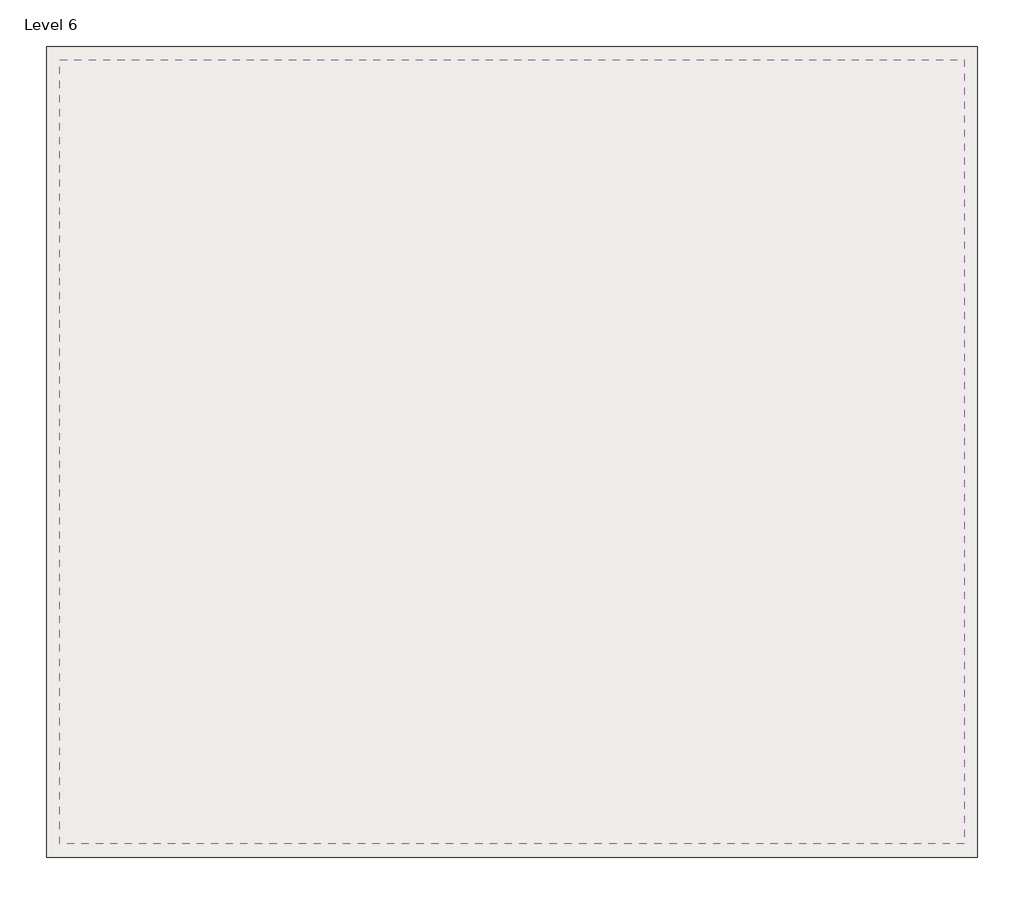
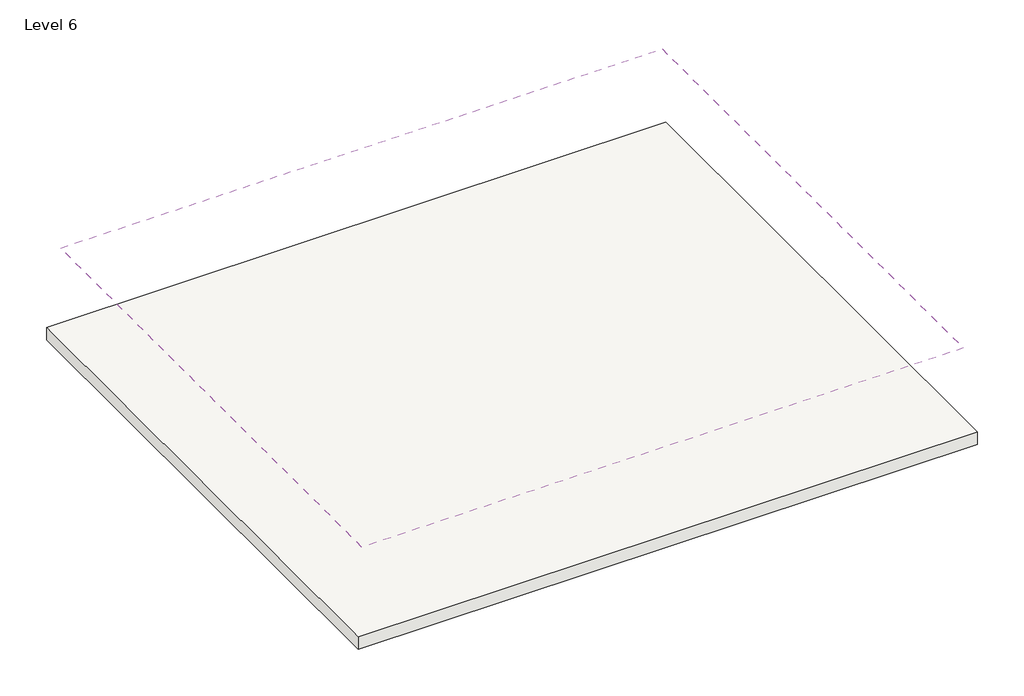
# One storey: 1 covering, 1 slab.
"""IFC4 building model written with IfcOpenShell, lengths in millimetres."""

from ifc_helpers import new_model, si_unit, frame, origin, place, context, project, spatial, polyline, outline, extrude, element, save

model = new_model("IFC4")

# Units and contexts
model_context = context("Model", 3, world=origin())
ifc_project = project(units=[si_unit("LENGTHUNIT", "METRE", prefix="MILLI")], contexts=[model_context])

# Site, building, storey
site = spatial("IfcSite", under=ifc_project)
building = spatial("IfcBuilding", under=site)
storey = spatial("IfcBuildingStorey", under=building, Name="Level 6", Elevation=15240.0)

# Covering
placement = place(None, origin())
element("IfcCovering", 1, ObjectType="2' x 4' ACT System", at=placement, inside=storey, context=model_context, shape_type="SweptSolid", body=[
    extrude(outline(polyline([(-12179.4937431, 6319.013611), (-9537.8937431, 6319.013611), (1638.1062569, 6319.013611), (1638.1062569, -2672.586389), (1638.1062569, -5669.786389), (-2527.4937431, -5669.786389), (-5270.6937431, -5669.786389), (-9537.8937431, -5669.786389), (-12179.4937431, -5669.786389), (-12179.4937431, -2723.386389), (-12179.4937431, 6319.013611)])), frame((0.0, 0.0, 17678.4), z_axis=(0.0, 0.0, 1.0), x_axis=(1.0, 0.0, 0.0)), (0.0, 0.0, 1.0), 57.15),
])

# Slab
element("IfcSlab", 2, ObjectType="Generic - 12\"", at=placement, inside=storey, context=model_context, shape_type="SweptSolid", body=[
    extrude(outline(polyline([(1841.3062569, 6522.213611), (1841.3062569, -5872.986389), (-12382.6937431, -5872.986389), (-12382.6937431, 6522.213611), (1841.3062569, 6522.213611)])), frame((0.0, 0.0, 15392.4), z_axis=(0.0, 0.0, 1.0), x_axis=(1.0, 0.0, 0.0)), (0.0, 0.0, 1.0), 304.8),
])

save(model, "model.ifc")

# Revit data of these elements
# Type "2' x 4' ACT System"
#   Assembly Code = "C3030210"
#   built-in parameter 1002203 = 1 (stored number, unit not read)
#   built-in parameter 1002202 = 1 (stored number, unit not read)
#   Layers, outside or top first: 0' - 1 5/8" "Default" (function 1); 0' - 0 5/8" "Acoustic Ceiling Tile 24 x 48" (function 5)
# Type "Generic - 12\""
#   Assembly Code = "B1010"
#   Function = 0
#   Layers, outside or top first: 1' - 0" "Parking Stripe" (function 1)
# Element 1 (IfcCovering, "2' x 4' ACT System")
#   Height Offset From Level = 8' - 0"
#   Phase Created = New Construction
#   Materials on its faces: "Acoustic Ceiling Tile 24 x 48", "Default"
# Element 2 (IfcSlab, "Generic - 12\"")
#   Height Offset From Level = 1' - 6"
#   Phase Created = New Construction
#   Materials on its faces: "Parking Stripe"
# Materials
#   "Default": colour RGB 127 127 127, transparency 0
#   "Acoustic Ceiling Tile 24 x 48": class "Generic", colour RGB 229 229 229, transparency 0, Description = "Acoustic Ceiling Tile 24 x 48", Cost = 0
#   "Parking Stripe": class "Paint", colour RGB 250 250 91, transparency 0, Cost = 0
